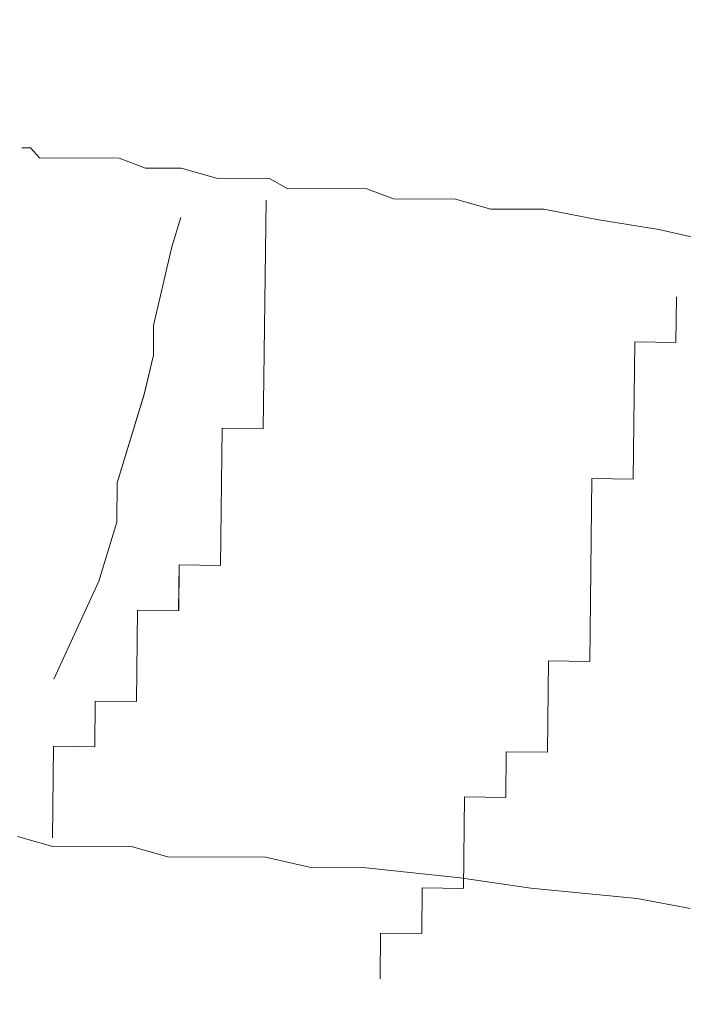
# Model space of a CAD drawing. Units: inches. Extents: x -466983 to 1020, y 324 to 318697.
# Tile 64 of 97: x 640.735 to 642.74, y 945.669 to 948.644. Entities that reach past the tile are written whole.
import ezdxf

# ---------------------------------------------------------------- set-up
doc = ezdxf.new("R2010")
doc.units = ezdxf.units.IN
doc.header["$MEASUREMENT"] = 0
doc.layers.add('A-FLOR-PATT', color=252, linetype='Continuous', lineweight=13)
doc.layers.add('A-FURN', color=8, linetype='Continuous', lineweight=18)

# ---------------------------------------------------------------- blocks, each defined once
blk = doc.blocks.new('L Shaped Sofa')
at = {"ltscale": 2}
for p, q in [((2422.3278, 737.9207), (2422.3309, 738.1726)), ((2422.0979, 737.6715), (2422.101, 737.9234)), ((2422.101, 737.9234), (2422.3278, 737.9207)), ((2420.6221, 737.7847), (2420.9145, 737.7291)), ((2420.9145, 737.7291), (2421.4997, 737.6721)), ((2421.4997, 737.6721), (2421.8898, 737.6161)), ((2421.8649, 737.1705), (2421.8711, 737.6743)), ((2421.8711, 737.6743), (2422.0979, 737.6715)), ((2421.8898, 737.6161), (2422.4262, 737.5593)), ((2422.4262, 737.5593), (2422.719, 737.558)), ((2422.719, 737.558), (2422.9626, 737.5026)), ((2422.9626, 737.5026), (2423.4994, 737.5001)), ((2423.4994, 737.5001), (2423.6942, 737.4449)), ((2423.6942, 737.4449), (2424.1334, 737.4429)), ((2424.1334, 737.4429), (2424.3282, 737.3878)), ((2424.1302, 736.8908), (2424.1364, 737.3947)), ((2421.635, 736.9213), (2421.6381, 737.1732)), ((2421.6381, 737.1732), (2421.8649, 737.1705)), ((2421.402, 736.4203), (2421.4082, 736.9241)), ((2421.4082, 736.9241), (2421.635, 736.9213)), ((2423.9003, 736.6417), (2423.9034, 736.8936)), ((2423.9034, 736.8936), (2424.1302, 736.8908)), ((2423.6673, 736.1406), (2423.6735, 736.6445)), ((2423.6735, 736.6445), (2423.9003, 736.6417)), ((2423.8804, 735.9802), (2424.1277, 736.5212)), ((2421.1629, 735.4154), (2421.1752, 736.423)), ((2421.1752, 736.423), (2421.402, 736.4203)), ((2423.4374, 735.8915), (2423.4405, 736.1434)), ((2423.4405, 736.1434), (2423.6673, 736.1406)), ((2423.7808, 735.6554), (2423.8804, 735.9802)), ((2423.2013, 735.1385), (2423.2106, 735.8943)), ((2423.2106, 735.8943), (2423.4374, 735.8915)), ((2423.7795, 735.4385), (2423.7808, 735.6554)), ((2420.9268, 734.6624), (2420.936, 735.4182)), ((2420.936, 735.4182), (2421.1629, 735.4154)), ((2423.6301, 734.9512), (2423.7795, 735.4385)), ((2422.9591, 733.8818), (2422.9745, 735.1413)), ((2422.9745, 735.1413), (2423.2013, 735.1385)), ((2423.58, 734.7346), (2423.6301, 734.9512)), ((2423.579, 734.572), (2423.58, 734.7346)), ((2420.6969, 734.4133), (2420.7, 734.6652)), ((2420.7, 734.6652), (2420.9268, 734.6624)), ((2423.4788, 734.1387), (2423.579, 734.572)), ((2423.429, 733.9763), (2423.4788, 734.1387)), ((2420.5507, 734.0982), (2420.7944, 734.0429)), ((2420.7944, 734.0429), (2421.1356, 733.987)), ((2421.1356, 733.987), (2421.428, 733.9315)), ((2421.428, 733.9315), (2421.7208, 733.9301)), ((2421.7208, 733.9301), (2421.9157, 733.8749)), ((2421.9157, 733.8749), (2422.2572, 733.8733)), ((2422.2572, 733.8733), (2422.4033, 733.8184)), ((2422.4033, 733.8184), (2422.8424, 733.8164)), ((2422.8424, 733.8164), (2422.9397, 733.7617)), ((2422.9397, 733.7617), (2423.2325, 733.7603)), ((2423.2325, 733.7603), (2423.4273, 733.7052)), ((2423.4273, 733.7052), (2423.6225, 733.7043)), ((2423.6225, 733.7043), (2423.7686, 733.6494)), ((2423.7686, 733.6494), (2424.2077, 733.6473)), ((2424.2077, 733.6473), (2424.2562, 733.5929)), ((2424.2562, 733.5929), (2424.305, 733.5926))]:
    blk.add_line(p, q, dxfattribs=at)

msp = doc.modelspace()

# ---------------------------------------------------------------- hatches: boundary and pattern name
at = {"layer": 'A-FLOR-PATT', "transparency": 33554572}
h = msp.add_hatch(dxfattribs=at)
h.set_pattern_fill('ANSI37', color=256, scale=30)
h.set_pattern_definition([(45, (-1212.4137, -290.035), (-2.6516504, 2.6516504), []), (135, (-1212.4137, -290.035), (-2.6516504, -2.6516504), [])])
h.paths.add_polyline_path([(901.8057, 1075.9377), (900.6144, 1075.9377), (900.6144, 1065.3856), (899.391, 1065.3856), (898.0911, 1065.3856), (892.8356, 1058.7098, -0.258377), (892.1875, 1058.3509), (879.9848, 1058.3509, -0.20177), (879.4382, 1058.5808), (874.0812, 1065.3856), (872.7813, 1065.3856), (871.5579, 1065.3856), (871.5579, 1075.9377), (813.8057, 1075.9377), (813.8057, 1044.7922), (832.3947, 1044.7922, -0.394795), (848.6602, 1028.5356), (848.6602, 1009.9377), (901.8057, 1009.9377), (901.8057, 1015.9377), (901.3057, 1015.9377), (871.3057, 1015.9377), (871.3057, 1017.2502), (871.3344, 1017.2502, -0.401453), (901.3057, 1045.9377), (901.8057, 1045.9377)])
edge = h.paths.add_edge_path(flags=16)
edge.add_line((847.7731, 1068.9486), (847.7731, 1073.7088))
edge.add_arc((849.2269, 1073.7088), 1.4538, 90, 180, ccw=False)
edge.add_line((849.2269, 1075.1627), (864.4921, 1075.1627))
edge.add_arc((864.4921, 1073.7088), 1.4538, 0, 90, ccw=False)
edge.add_line((865.9459, 1073.7088), (865.9459, 1069.0035))
edge.add_arc((832.6447, 1068.9761), 33.3012, -20.61234, 0.04725, ccw=False)
edge.add_ellipse((856.8595, 1058.48), major_axis=(0, 10.2131), ratio=0.6859192, start_angle=100.00884, end_angle=259.99116, ccw=False)
edge.add_arc((881.0742, 1068.9761), 33.3012, 180.04725, 200.61234, ccw=False)
h.paths.add_polyline_path([(853.1456, 1066.4815), (853.1456, 1066.4534), (853.1463, 1066.4534, 0.433107), (852.9166, 1066.6849), (852.9166, 1066.4534), (853.1456, 1066.4534), (853.1456, 1066.4815), (853.088, 1066.6122, 0.697939), (852.6995, 1066.4534), (852.7003, 1066.4534), (852.7003, 1066.4815), (852.9166, 1067.0012), (852.9166, 1066.6849, -0.396254)], flags=0)
h.paths.add_polyline_path([(861.0187, 1066.4815), (861.0187, 1066.4534), (861.0194, 1066.4534, 0.416404), (860.8024, 1066.6849), (860.8024, 1066.4534), (861.0187, 1066.4534), (861.0187, 1066.4815), (860.9672, 1066.6053, 0.713344), (860.5726, 1066.4534), (860.5734, 1066.4534), (860.5734, 1066.4815), (860.8024, 1067.0012), (860.8024, 1066.6849, -0.379973)], flags=0)
edge = h.paths.add_edge_path(flags=0)
edge.add_spline(control_points=[(861.1298, 1065.7855), (861.4661, 1065.2478), (861.6134, 1065.0161), (861.9833, 1064.3736), (862.1924, 1063.9443), (862.5614, 1063.0391), (862.7212, 1062.5633), (862.9865, 1061.5781), (863.092, 1061.0689), (863.2452, 1060.031), (863.293, 1059.5025), (863.3295, 1058.4409), (863.3181, 1057.9078), (863.2366, 1056.8518), (863.1664, 1056.3289), (862.9695, 1055.308), (862.8427, 1054.8099), (862.5365, 1053.8522), (862.3571, 1053.3927), (861.9514, 1052.5249), (861.7251, 1052.1166), (861.233, 1051.3622), (860.9672, 1051.0162), (860.4048, 1050.3949), (860.1082, 1050.1197), (859.4937, 1049.6461), (859.1758, 1049.4476), (858.5276, 1049.1299), (858.1973, 1049.0107), (857.5315, 1048.8518), (857.1959, 1048.8121), (856.5249, 1048.812), (856.1894, 1048.8515), (855.5236, 1049.0101), (855.1933, 1049.1291), (854.545, 1049.4465), (854.2271, 1049.6449), (853.6124, 1050.1183), (853.3158, 1050.3933), (852.7533, 1051.0143), (852.4874, 1051.3602), (851.9952, 1052.1144), (851.7688, 1052.5225), (851.3629, 1053.3902), (851.1834, 1053.8496), (850.877, 1054.8071), (850.7501, 1055.3051), (850.553, 1056.326), (850.4827, 1056.8488), (850.401, 1057.9048), (850.3895, 1058.4379), (850.4257, 1059.4995), (850.4734, 1060.0281), (850.6265, 1061.066), (850.7318, 1061.5753), (850.9969, 1062.5605), (851.1567, 1063.0365), (851.5254, 1063.9418), (851.7345, 1064.3712), (852.1056, 1065.0164), (852.2544, 1065.2503), (852.6082, 1065.7335)], knot_values=[3.915332, 3.915332, 3.915332, 3.915332, 4.013468, 4.013468, 4.175532, 4.175532, 4.337596, 4.337596, 4.49966, 4.49966, 4.661724, 4.661724, 4.823788, 4.823788, 4.985852, 4.985852, 5.147916, 5.147916, 5.30998, 5.30998, 5.472044, 5.472044, 5.634109, 5.634109, 5.796173, 5.796173, 5.958237, 5.958237, 6.120301, 6.120301, 6.282365, 6.282365, 6.444429, 6.444429, 6.606493, 6.606493, 6.768557, 6.768557, 6.930621, 6.930621, 7.092685, 7.092685, 7.254749, 7.254749, 7.416813, 7.416813, 7.578878, 7.578878, 7.740942, 7.740942, 7.903006, 7.903006, 8.06507, 8.06507, 8.227134, 8.227134, 8.389198, 8.389198, 8.551262, 8.551262, 8.65037, 8.65037, 8.65037, 8.65037], degree=3, periodic=0)
edge.add_line((852.6421, 1065.7855), (861.1298, 1065.7855))
edge = h.paths.add_edge_path(flags=0)
edge.add_ellipse((856.8496, 1057.7432), major_axis=(0, 7.7921), ratio=0.687861, start_angle=0, end_angle=360)
h.paths.add_polyline_path([(848.8634, 1069.3891), (848.8634, 1073.9605, -0.414214), (849.9538, 1075.0508), (863.7652, 1075.0508, -0.414214), (864.8555, 1073.9605), (864.8555, 1069.3891, -0.388936), (864.5237, 1069.027, -0.043561), (849.1953, 1069.027, -0.388936)], flags=0)
h.paths.add_polyline_path([(853.1006, 1068.1122, -1), (852.6775, 1068.1122, -1)], flags=0)
edge = h.paths.add_edge_path(flags=0)
edge.add_ellipse((856.8595, 1057.3378), major_axis=(0, 2.207), ratio=0.657164, start_angle=0, end_angle=360)
h.paths.add_polyline_path([(861.0415, 1068.1122, -1), (860.6184, 1068.1122, -1)], flags=0)
edge = h.paths.add_edge_path()
edge.add_line((573.9537, 1057.3412), (573.9537, 1075.9377))
edge.add_line((573.9537, 1075.9377), (558.7308, 1075.9377))
edge.add_line((558.7308, 1075.9377), (558.7308, 1065.3856))
edge.add_line((558.7308, 1065.3856), (557.5074, 1065.3856))
edge.add_line((557.5074, 1065.3856), (556.2075, 1065.3856))
edge.add_line((556.2075, 1065.3856), (550.952, 1058.7098))
edge.add_arc((550.3039, 1059.1155), 0.7646, 270, 327.9483, ccw=False)
edge.add_line((550.3039, 1058.3509), (538.1012, 1058.3509))
edge.add_arc((538.1012, 1059.1155), 0.7646, 224.3704, 270, ccw=False)
edge.add_line((537.5546, 1058.5808), (532.1976, 1065.3856))
edge.add_line((532.1976, 1065.3856), (530.8977, 1065.3856))
edge.add_line((530.8977, 1065.3856), (529.6743, 1065.3856))
edge.add_line((529.6743, 1065.3856), (529.6743, 1075.9377))
edge.add_line((529.6743, 1075.9377), (520.8057, 1075.9377))
edge.add_line((520.8057, 1075.9377), (520.8057, 1045.9377))
edge.add_line((520.8057, 1045.9377), (521.3057, 1045.9377))
edge.add_arc((521.3057, 1015.9377), 30, 2.50749, 90, ccw=False)
edge.add_line((551.277, 1017.2502), (551.3057, 1017.2502))
edge.add_line((551.3057, 1017.2502), (551.3057, 1015.9377))
edge.add_line((551.3057, 1015.9377), (520.8057, 1015.9377))
edge.add_line((520.8057, 1015.9377), (520.8057, 1009.9377))
edge.add_line((520.8057, 1009.9377), (559.1913, 1010.4022))
edge.add_arc((559.1913, 1011.856), 1.4538, 180, 270, ccw=False)
edge.add_line((557.7375, 1011.856), (557.7375, 1016.5613))
edge.add_arc((591.0386, 1016.5888), 33.3012, 159.38766, 180.04725, ccw=False)
edge.add_ellipse((566.8239, 1027.0848), major_axis=(0, 10.2131), ratio=0.6859192, start_angle=280.00884, end_angle=439.99116, ccw=False)
edge.add_arc((542.6091, 1016.5888), 33.3012, 0.04725, 20.61234, ccw=False)
edge.add_line((575.9103, 1016.6162), (575.9103, 1011.856))
edge.add_arc((574.4565, 1011.856), 1.4538, -90, 0, ccw=False)
edge.add_line((574.4565, 1010.4022), (608.8057, 1009.9377))
edge.add_line((608.8057, 1009.9377), (608.8057, 1041.0857))
edge.add_line((608.8057, 1041.0857), (590.2179, 1041.0857))
edge.add_arc((590.775, 1057.9074), 16.8309, 181.92775, 268.10321, ccw=False)
edge = h.paths.add_edge_path()
edge.add_ellipse((494.2443, 583.6204), major_axis=(0, 10.2131), ratio=0.6859192, start_angle=280.00884, end_angle=439.99116, ccw=False)
edge.add_arc((470.0296, 573.1243), 33.3012, 0.04725, 20.61234, ccw=False)
edge.add_line((503.3307, 573.1518), (503.3307, 568.3916))
edge.add_arc((501.8769, 568.3916), 1.4538, -90, 0, ccw=False)
edge.add_line((501.8769, 566.9377), (539.8057, 566.9377))
edge.add_line((539.8057, 566.9377), (539.8057, 572.9377))
edge.add_line((539.8057, 572.9377), (539.3057, 572.9377))
edge.add_line((539.3057, 572.9377), (509.3057, 572.9377))
edge.add_line((509.3057, 572.9377), (509.3057, 574.2502))
edge.add_line((509.3057, 574.2502), (509.3344, 574.2502))
edge.add_arc((539.3057, 572.9377), 30, 90, 177.49251, ccw=False)
edge.add_line((539.3057, 602.9377), (539.8057, 602.9377))
edge.add_line((539.8057, 602.9377), (539.8057, 626.9377))
edge.add_line((539.8057, 626.9377), (531.7718, 626.9377))
edge.add_line((531.7718, 626.9377), (531.7718, 616.3856))
edge.add_line((531.7718, 616.3856), (530.5484, 616.3856))
edge.add_line((530.5484, 616.3856), (529.2485, 616.3856))
edge.add_line((529.2485, 616.3856), (523.7105, 609.3509))
edge.add_line((523.7105, 609.3509), (510.7766, 609.3509))
edge.add_line((510.7766, 609.3509), (505.2386, 616.3856))
edge.add_line((505.2386, 616.3856), (503.9387, 616.3856))
edge.add_line((503.9387, 616.3856), (502.7153, 616.3856))
edge.add_line((502.7153, 616.3856), (502.7153, 626.9377))
edge.add_line((502.7153, 626.9377), (481.6983, 626.9377))
edge.add_line((481.6983, 626.9377), (481.6983, 610.995))
edge.add_arc((467.2703, 611.4728), 14.4359, 271.92775, 358.10321, ccw=False)
edge.add_line((467.7559, 597.0451), (451.8057, 597.0451))
edge.add_line((451.8057, 597.0451), (451.8057, 584.4035))
edge.add_line((451.8057, 584.4035), (451.8057, 566.9377))
edge.add_line((451.8057, 566.9377), (486.6117, 566.9377))
edge.add_arc((486.6117, 568.3916), 1.4538, 180, 270, ccw=False)
edge.add_line((485.1579, 568.3916), (485.1579, 573.0969))
edge.add_arc((518.4591, 573.1243), 33.3012, 159.38766, 180.04725, ccw=False)
h.paths.add_polyline_path([(836.2609, 1020.7328), (879.8898, 1020.7328), (879.8898, 1039.3902), (836.2609, 1039.3902)], flags=25)
h.paths.add_polyline_path([(549.9851, 1036.7492), (593.614, 1036.7492), (593.614, 1055.4065), (549.9851, 1055.4065)], flags=24)
h.paths.add_polyline_path([(475.123, 595.5959), (518.752, 595.5959), (518.752, 614.2532), (475.123, 614.2532)], flags=24)
h = msp.add_hatch(dxfattribs=at)
h.set_pattern_fill('ANSI37', color=256, scale=20)
h.set_pattern_definition([(45, (-1212.4137, -290.035), (-1.767767, 1.767767), []), (135, (-1212.4137, -290.035), (-1.767767, -1.767767), [])])
h.paths.add_polyline_path([(809.8057, 870.9377), (809.8057, 888.1519), (806.9985, 888.1519), (802.6624, 888.1519), (789.3832, 888.1519), (786.2846, 888.1519, -0.414214), (785.4991, 888.9374), (785.4991, 900.1959), (785.4991, 908.4696, -0.414214), (786.8082, 909.7787, -0.414214), (785.4991, 911.0878), (785.4991, 929.1015, -0.414214), (786.8082, 930.4106, -0.414214), (785.4991, 931.7197), (785.4991, 931.9039, -0.414214), (784.19, 930.5948), (766.7223, 930.5948, -0.412359), (765.4132, 931.8956, -0.413741), (764.1145, 930.5782), (744.5781, 930.422, -0.416556), (743.7864, 931.2075), (743.7864, 933.5153), (742.2154, 933.5153), (742.2154, 952.024, -0.001344), (743.7864, 952.1998), (743.7864, 953.9377), (678.5915, 953.9377), (678.5915, 951.1305), (678.5915, 946.7945), (678.5915, 933.5153), (678.5915, 930.4166, -0.414214), (677.806, 929.6312), (666.5475, 929.6312), (658.2738, 929.6312, -0.414214), (656.9647, 930.9403, -0.414214), (655.6556, 929.6312), (637.6419, 929.6312, -0.414214), (636.3328, 930.9403, -0.414214), (635.0237, 929.6312), (634.8395, 929.6312, -0.414214), (636.1486, 928.322), (636.1486, 910.8544, -0.412359), (634.8478, 909.5452, -0.413741), (636.1653, 908.2466), (636.3214, 888.7102, -0.416556), (635.5359, 887.9184), (633.2281, 887.9184), (633.2281, 886.3475), (614.7194, 886.3475, -0.001344), (614.5436, 887.9184), (612.8057, 887.9184), (612.8057, 834.9377), (612.8057, 752.9377), (612.8057, 748.9377), (612.8057, 697.9377), (654.8057, 697.9377), (654.8057, 701.9377), (715.8057, 701.9377), (715.8057, 737.4353), (774.2918, 737.4353), (774.2918, 795.9377), (809.8057, 795.9377)])
h.paths.add_polyline_path([(679.2761, 849.5757, 0.102523), (682.1475, 849.2608, -0.080461), (694.5428, 849.7725, -0.283899), (694.4822, 849.0082, 0.136605), (694.4068, 848.8103, -0.030441), (694.5428, 846.8929), (694.5428, 842.6198), (694.5428, 838.3466, -0.028219), (694.4246, 836.5684), (694.425, 836.5684, 0.196187), (694.4456, 836.2708, -0.302897), (694.5428, 835.467, -0.080461), (682.1475, 835.9787, 0.102523), (679.2761, 835.6638, -0.58611), (678.6457, 836.0169), (678.6457, 849.2227, -0.58611)], flags=16)
h.paths.add_polyline_path([(679.5173, 848.6515, 0.699597), (679.476, 848.6342, 1.20716), (679.1935, 848.7422, 0.010621)], flags=0)
h.paths.add_polyline_path([(679.4923, 836.5608, -0.013798), (679.9178, 836.6594, -0.071703), (682.8533, 837.1434, -0.165743), (682.1665, 839.1006), (682.1665, 842.6094), (682.1665, 846.0603, -0.240616), (683.4733, 848.6767, -0.068263), (693.9295, 849.0082), (693.7875, 848.7083), (693.7875, 849.0228, 0.067332), (683.4733, 848.6767, 0.240616), (682.1665, 846.0603), (682.1665, 842.6094), (682.1665, 839.1006, 0.23459), (683.461, 836.5513, 0.068093), (693.7875, 836.1955), (693.7875, 836.5104), (693.9296, 836.2102, -0.077215), (682.2421, 836.7815, 0.086627), (679.5283, 836.5701, -0.628402), (679.5029, 836.5735), (679.5029, 836.6071, 0.910458)], flags=0)
h.paths.add_polyline_path([(679.476, 848.6364), (679.2069, 848.647), (679.2069, 836.5718, 0.913566), (679.3645, 836.5861), (679.476, 836.5824)], flags=0)
h.paths.add_polyline_path([(679.2761, 829.8604, 0.102523), (682.1475, 829.5455, -0.080461), (694.5428, 830.0572, -0.283899), (694.4822, 829.2929, 0.136605), (694.4068, 829.095, -0.030441), (694.5428, 827.1776), (694.5428, 822.9045), (694.5428, 818.6314, -0.028219), (694.4246, 816.8531), (694.425, 816.8532, 0.196187), (694.4456, 816.5555, -0.302897), (694.5428, 815.7517, -0.080461), (682.1475, 816.2635, 0.102523), (679.2761, 815.9485, -0.58611), (678.6457, 816.3016), (678.6457, 829.5074, -0.58611)], flags=16)
h.paths.add_polyline_path([(679.5173, 828.9362, 0.699597), (679.476, 828.9189, 1.20716), (679.1935, 829.0269, 0.010621)], flags=0)
h.paths.add_polyline_path([(679.4923, 816.8456, -0.013798), (679.9178, 816.9441, -0.071703), (682.8533, 817.4281, -0.165743), (682.1665, 819.3853), (682.1665, 822.8941), (682.1665, 826.345, -0.240616), (683.4733, 828.9614, -0.068263), (693.9295, 829.2929), (693.7875, 828.9931), (693.7875, 829.3076, 0.067332), (683.4733, 828.9614, 0.240616), (682.1665, 826.345), (682.1665, 822.8941), (682.1665, 819.3853, 0.23459), (683.461, 816.836, 0.068093), (693.7875, 816.4802), (693.7875, 816.7952), (693.9296, 816.4949, -0.077215), (682.2421, 817.0662, 0.086627), (679.5283, 816.8549, -0.628402), (679.5029, 816.8582), (679.5029, 816.8918, 0.910458)], flags=0)
h.paths.add_polyline_path([(679.476, 828.9211), (679.2069, 828.9317), (679.2069, 816.8565, 0.913566), (679.3645, 816.8708), (679.476, 816.8671)], flags=0)
h.paths.add_polyline_path([(679.2761, 810.1451, 0.102523), (682.1475, 809.8302, -0.080461), (694.5428, 810.342, -0.3023), (694.4466, 809.5394, 0.10023), (694.4058, 809.3878, -0.03057), (694.5428, 807.4623), (694.5428, 803.1892), (694.5428, 798.9161, -0.03057), (694.4058, 796.9906, 0.10023), (694.4466, 796.839, -0.3023), (694.5428, 796.0365, -0.080461), (682.1475, 796.5482, 0.102523), (679.2761, 796.2333, -0.58611), (678.6457, 796.5863), (678.6457, 809.7921, -0.58611)], flags=16)
h.paths.add_polyline_path([(679.5173, 809.2417, 0.699597), (679.476, 809.2244, 1.20716), (679.1935, 809.3324, 0.010621)], flags=0)
h.paths.add_polyline_path([(679.4923, 797.151, -0.013798), (679.9178, 797.2496, -0.071703), (682.8533, 797.7336, -0.165743), (682.1665, 799.6908), (682.1665, 803.1996), (682.1665, 806.6505, -0.239349), (683.461, 809.2577, -0.072465), (694.4468, 809.5405, 0.197932), (694.425, 809.2405), (693.7875, 809.2985), (693.7875, 809.6135, 0.068093), (683.461, 809.2577, 0.239349), (682.1665, 806.6505), (682.1665, 803.1996), (682.1665, 799.6908, 0.235854), (683.4733, 797.1323, 0.067332), (693.7875, 796.7861), (693.7875, 797.1006), (694.425, 797.1586, 0.197932), (694.4468, 796.8586, -0.080419), (682.1557, 797.3795, 0.083867), (679.5283, 797.1603, -0.628402), (679.5029, 797.1637), (679.5029, 797.1973, 0.910458)], flags=0)
h.paths.add_polyline_path([(679.2069, 809.2372), (679.2069, 797.162, 0.913566), (679.3645, 797.1763), (679.476, 797.1726), (679.476, 809.2266)], flags=0)
h.paths.add_polyline_path([(695.3643, 853.2989), (728.2231, 853.2989), (728.2231, 771.1519), (695.3643, 771.1519)], flags=16)
h.paths.add_polyline_path([(696.0215, 852.6417), (727.5659, 852.6417), (727.5659, 771.809), (696.0215, 771.809)], flags=0)
h.paths.add_polyline_path([(679.2761, 788.7869, 0.102523), (682.1475, 788.472, -0.080461), (694.5428, 788.9837, -0.3023), (694.4466, 788.1812, 0.10023), (694.4058, 788.0296, -0.03057), (694.5428, 786.1041), (694.5428, 781.831), (694.5428, 777.5578, -0.03057), (694.4058, 775.6323, 0.10023), (694.4466, 775.4808, -0.3023), (694.5428, 774.6782, -0.080461), (682.1475, 775.19, 0.102523), (679.2761, 774.875, -0.58611), (678.6457, 775.2281), (678.6457, 788.4339, -0.58611)], flags=16)
h.paths.add_polyline_path([(679.5173, 787.8834, 0.699597), (679.476, 787.8662, 1.20716), (679.1935, 787.9742, 0.010621)], flags=0)
h.paths.add_polyline_path([(679.4923, 775.7928, -0.013798), (679.9178, 775.8914, -0.071703), (682.8533, 776.3753, -0.165743), (682.1665, 778.3325), (682.1665, 781.8414), (682.1665, 785.2922, -0.239349), (683.461, 787.8995, -0.072465), (694.4468, 788.1823, 0.197932), (694.425, 787.8823), (693.7875, 787.9403), (693.7875, 788.2553, 0.068093), (683.461, 787.8995, 0.239349), (682.1665, 785.2922), (682.1665, 781.8414), (682.1665, 778.3325, 0.235854), (683.4733, 775.7741, 0.067332), (693.7875, 775.4279), (693.7875, 775.7424), (694.425, 775.8004, 0.197932), (694.4468, 775.5004, -0.080419), (682.1557, 776.0212, 0.083867), (679.5283, 775.8021, -0.628402), (679.5029, 775.8054), (679.5029, 775.8391, 0.910458)], flags=0)
h.paths.add_polyline_path([(679.2069, 787.8789), (679.2069, 775.8038, 0.913566), (679.3645, 775.818), (679.476, 775.8144), (679.476, 787.8684)], flags=0)
h.paths.add_polyline_path([(704.641, 854.1204, -0.080461), (705.1527, 866.5157, 0.102523), (704.8378, 869.3871, -0.58611), (705.1908, 870.0174), (718.3966, 870.0174, -0.58611), (718.7496, 869.3871, 0.102523), (718.4347, 866.5157, -0.080461), (718.9465, 854.1204, -0.3023), (718.1439, 854.2166, 0.10023), (717.9924, 854.2574, -0.03057), (716.0668, 854.1204), (711.7937, 854.1204), (707.5206, 854.1204, -0.03057), (705.5951, 854.2574, 0.10023), (705.4435, 854.2166, -0.3023)], flags=16)
h.paths.add_polyline_path([(717.8462, 869.1459, 0.699597), (717.8289, 869.1872, 1.20716), (717.9369, 869.4697, 0.010621)], flags=0)
h.paths.add_polyline_path([(705.4631, 854.2164, -0.080419), (705.984, 866.5074, 0.083867), (705.7648, 869.1349, -0.628402), (705.7682, 869.1603), (705.8018, 869.1603, 0.910458), (705.7555, 869.1709, -0.013798), (705.8541, 868.7454, -0.071703), (706.3381, 865.8099, -0.165743), (708.2953, 866.4967), (711.8041, 866.4967), (715.255, 866.4967, -0.239349), (717.8622, 865.2022, -0.072465), (718.145, 854.2164, 0.197932), (717.845, 854.2382), (717.903, 854.8757), (718.218, 854.8757, 0.068093), (717.8622, 865.2022, 0.239349), (715.255, 866.4967), (711.8041, 866.4967), (708.2953, 866.4967, 0.235854), (705.7368, 865.1898, 0.067332), (705.3906, 854.8757), (705.7051, 854.8757), (705.7631, 854.2382, 0.197932)], flags=16)
h.paths.add_polyline_path([(705.7665, 869.4563, 0.913566), (705.7808, 869.2987), (705.7771, 869.1872), (717.8311, 869.1872), (717.8417, 869.4563)], flags=0)
h.paths.add_polyline_path([(729.0446, 842.6198), (729.0446, 846.8929, -0.03057), (729.1817, 848.8184, 0.10023), (729.1408, 848.9699, -0.3023), (729.0446, 849.7725, -0.080461), (741.4399, 849.2608, 0.102523), (744.3113, 849.5757, -0.58611), (744.9417, 849.2227), (744.9417, 836.0169, -0.58611), (744.3113, 835.6638, 0.102523), (741.4399, 835.9787, -0.080461), (729.0446, 835.467, -0.3023), (729.1408, 836.2696, 0.10023), (729.1817, 836.4211, -0.03057), (729.0446, 838.3466)], flags=16)
h.paths.add_polyline_path([(744.1115, 836.5846, 1.20716), (744.3939, 836.4766, 0.010621), (744.0701, 836.5673, 0.699597)], flags=0)
h.paths.add_polyline_path([(729.1407, 836.2684, 0.197932), (729.1624, 836.5684), (729.7999, 836.5104), (729.7999, 836.1955, 0.068093), (740.1264, 836.5513, 0.239349), (741.4209, 839.1585), (741.4209, 842.6094), (741.4209, 846.1182, 0.235854), (740.1141, 848.6767, 0.067332), (729.7999, 849.0228), (729.7999, 848.7083), (729.1624, 848.6503, 0.197932), (729.1407, 848.9504, -0.080419), (741.4317, 848.4295, 0.083867), (744.0591, 848.6486, -0.628402), (744.0845, 848.6453), (744.0845, 848.6117, 0.910458), (744.0951, 848.6579, -0.013798), (743.6696, 848.5594, -0.071703), (740.7341, 848.0754, -0.165743), (741.4209, 846.1182), (741.4209, 842.6094), (741.4209, 839.1585, -0.239349), (740.1264, 836.5513, -0.072465)], flags=0)
h.paths.add_polyline_path([(729.0446, 830.0572, -0.080461), (741.4399, 829.5455, 0.102523), (744.3113, 829.8604, -0.58611), (744.9417, 829.5074), (744.9417, 816.3016, -0.58611), (744.3113, 815.9485, 0.102523), (741.4399, 816.2635, -0.080461), (729.0446, 815.7517, -0.3023), (729.1408, 816.5543, 0.10023), (729.1817, 816.7058, -0.03057), (729.0446, 818.6314), (729.0446, 822.9045), (729.0446, 827.1776, -0.03057), (729.1817, 829.1031, 0.10023), (729.1408, 829.2547, -0.3023)], flags=16)
h.paths.add_polyline_path([(744.1115, 816.8693, 1.20716), (744.3939, 816.7613, 0.010621), (744.0701, 816.852, 0.699597)], flags=0)
h.paths.add_polyline_path([(729.1407, 829.2351, -0.080419), (741.4317, 828.7142, 0.083867), (744.0591, 828.9334, -0.628402), (744.0845, 828.93), (744.0845, 828.8964, 0.910458), (744.0951, 828.9427, -0.013798), (743.6696, 828.8441, -0.071703), (740.7341, 828.3601, -0.165743), (741.4209, 826.4029), (741.4209, 822.8941), (741.4209, 819.4432, -0.239349), (740.1264, 816.836, -0.072465), (729.1407, 816.5531, 0.197932), (729.1624, 816.8532), (729.7999, 816.7952), (729.7999, 816.4802, 0.068093), (740.1264, 816.836, 0.239349), (741.4209, 819.4432), (741.4209, 822.8941), (741.4209, 826.4029, 0.235854), (740.1141, 828.9614, 0.067332), (729.7999, 829.3076), (729.7999, 828.9931), (729.1624, 828.9351, 0.197932)], flags=16)
h.paths.add_polyline_path([(729.0446, 810.342, -0.080461), (741.4399, 809.8302, 0.102523), (744.3113, 810.1451, -0.58611), (744.9417, 809.7921), (744.9417, 796.5863, -0.58611), (744.3113, 796.2333, 0.102523), (741.4399, 796.5482, -0.080461), (729.0446, 796.0365, -0.283899), (729.1052, 796.8007, 0.136605), (729.1806, 796.9987, -0.030441), (729.0446, 798.9161), (729.0446, 803.1892), (729.0446, 807.4623, -0.028219), (729.1628, 809.2406), (729.1624, 809.2405, 0.196187), (729.1418, 809.5382, -0.302897)], flags=16)
h.paths.add_polyline_path([(744.1115, 797.1748, 1.20716), (744.3939, 797.0668, 0.010621), (744.0701, 797.1575, 0.699597)], flags=0)
h.paths.add_polyline_path([(741.3453, 809.0275, 0.086627), (744.0591, 809.2388, -0.628402), (744.0845, 809.2355), (744.0845, 809.2019, 0.910458), (744.0951, 809.2481, -0.013798), (743.6696, 809.1496, -0.071703), (740.7341, 808.6656, -0.165743), (741.4209, 806.7084), (741.4209, 803.1996), (741.4209, 799.7487, -0.240616), (740.1141, 797.1323, -0.068263), (729.658, 796.8008), (729.7999, 797.1006), (729.7999, 796.7861, 0.067332), (740.1141, 797.1323, 0.240616), (741.4209, 799.7487), (741.4209, 803.1996), (741.4209, 806.7084, 0.23459), (740.1264, 809.2577, 0.068093), (729.7999, 809.6135), (729.7999, 809.2985), (729.6578, 809.5988, -0.077215)], flags=0)
h.paths.add_polyline_path([(704.641, 770.3304, -0.283899), (705.4053, 770.2697, 0.136605), (705.6032, 770.1944, -0.030441), (707.5206, 770.3304), (711.7937, 770.3304), (716.0668, 770.3304, -0.028219), (717.8451, 770.2122), (717.845, 770.2126, 0.196187), (718.1427, 770.2331, -0.302897), (718.9465, 770.3304, -0.080461), (718.4347, 757.9351, 0.102523), (718.7496, 755.0637, -0.58611), (718.3966, 754.4333), (705.1908, 754.4333, -0.58611), (704.8378, 755.0637, 0.102523), (705.1527, 757.9351, -0.080461)], flags=16)
h.paths.add_polyline_path([(705.762, 755.3048, 0.699597), (705.7793, 755.2635, 1.20716), (705.6713, 754.9811, 0.010621)], flags=0)
h.paths.add_polyline_path([(705.4053, 769.717), (705.7051, 769.5751), (705.3906, 769.5751, 0.067332), (705.7368, 759.2609, 0.240616), (708.3532, 757.954), (711.8041, 757.954), (715.3129, 757.954, 0.23459), (717.8622, 759.2485, 0.068093), (718.218, 769.5751), (717.903, 769.5751), (718.2033, 769.7172, -0.077215), (717.632, 758.0297, 0.086627), (717.8433, 755.3159, -0.628402), (717.84, 755.2904), (717.8064, 755.2904, 0.910458), (717.8526, 755.2799, -0.013798), (717.7541, 755.7053, -0.071703), (717.2701, 758.6409, -0.165743), (715.3129, 757.954), (711.8041, 757.954), (708.3532, 757.954, -0.240616), (705.7368, 759.2609, -0.068263)], flags=0)
h.paths.add_polyline_path([(729.0446, 788.9837, -0.080461), (741.4399, 788.472, 0.102523), (744.3113, 788.7869, -0.58611), (744.9417, 788.4339), (744.9417, 775.2281, -0.58611), (744.3113, 774.875, 0.102523), (741.4399, 775.19, -0.080461), (729.0446, 774.6782, -0.283899), (729.1052, 775.4425, 0.136605), (729.1806, 775.6405, -0.030441), (729.0446, 777.5578), (729.0446, 781.831), (729.0446, 786.1041, -0.028219), (729.1628, 787.8823), (729.1624, 787.8823, 0.196187), (729.1418, 788.1799, -0.302897)], flags=16)
h.paths.add_polyline_path([(744.1115, 775.8165, 1.20716), (744.3939, 775.7086, 0.010621), (744.0701, 775.7993, 0.699597)], flags=0)
h.paths.add_polyline_path([(741.3453, 787.6692, 0.086627), (744.0591, 787.8806, -0.628402), (744.0845, 787.8773), (744.0845, 787.8437, 0.910458), (744.0951, 787.8899, -0.013798), (743.6696, 787.7913, -0.071703), (740.7341, 787.3074, -0.165743), (741.4209, 785.3502), (741.4209, 781.8414), (741.4209, 778.3905, -0.240616), (740.1141, 775.7741, -0.068263), (729.658, 775.4425), (729.7999, 775.7424), (729.7999, 775.4279, 0.067332), (740.1141, 775.7741, 0.240616), (741.4209, 778.3905), (741.4209, 781.8414), (741.4209, 785.3502, 0.23459), (740.1264, 787.8995, 0.068093), (729.7999, 788.2553), (729.7999, 787.9403), (729.6578, 788.2405, -0.077215)], flags=0)
h.paths.add_polyline_path([(744.1115, 848.6364), (744.1115, 836.5824), (744.3805, 836.5718), (744.3805, 848.647, 0.913566), (744.2229, 848.6327)], flags=0)
h.paths.add_polyline_path([(744.2229, 828.9174), (744.1115, 828.9211), (744.1115, 816.8671), (744.3805, 816.8565), (744.3805, 828.9317, 0.913566)], flags=0)
h.paths.add_polyline_path([(717.8311, 755.2635), (705.7771, 755.2635), (705.7665, 754.9945), (717.8417, 754.9945, 0.913566), (717.8274, 755.1521)], flags=0)
h.paths.add_polyline_path([(744.2229, 809.2229), (744.1115, 809.2266), (744.1115, 797.1726), (744.3805, 797.162), (744.3805, 809.2372, 0.913566)], flags=0)
h.paths.add_polyline_path([(744.1115, 787.8684), (744.1115, 775.8144), (744.3805, 775.8038), (744.3805, 787.8789, 0.913566), (744.2229, 787.8647)], flags=0)
h.paths.add_polyline_path([(678.8774, 877.1228), (737.6127, 877.1228), (737.6127, 899.5116), (678.8774, 899.5116)], flags=24)

# ---------------------------------------------------------------- linework, layer by layer
at = {"layer": 'A-FURN', "ltscale": 2}
for p, q in [((640.7683, 948.2563), (640.7415, 948.2564)), ((640.7683, 948.2563), (640.7415, 948.2564)), ((640.7683, 948.2563), (640.7415, 948.2564)), ((640.7683, 948.2563), (640.7415, 948.2564)), ((640.7683, 948.2563), (640.7415, 948.2564)), ((640.7683, 948.2563), (640.7415, 948.2564)), ((640.7949, 948.2265), (640.7683, 948.2563)), ((640.7949, 948.2265), (640.7683, 948.2563)), ((640.7949, 948.2265), (640.7683, 948.2563)), ((640.7949, 948.2265), (640.7683, 948.2563)), ((640.7949, 948.2265), (640.7683, 948.2563)), ((640.7949, 948.2265), (640.7683, 948.2563)), ((641.0356, 948.2253), (640.7949, 948.2265)), ((641.0356, 948.2253), (640.7949, 948.2265)), ((641.0356, 948.2253), (640.7949, 948.2265)), ((641.0356, 948.2253), (640.7949, 948.2265)), ((641.0356, 948.2253), (640.7949, 948.2265)), ((641.0356, 948.2253), (640.7949, 948.2265)), ((641.1157, 948.1952), (641.0356, 948.2253)), ((641.1157, 948.1952), (641.0356, 948.2253)), ((641.1157, 948.1952), (641.0356, 948.2253)), ((641.1157, 948.1952), (641.0356, 948.2253)), ((641.1157, 948.1952), (641.0356, 948.2253)), ((641.1157, 948.1952), (641.0356, 948.2253)), ((641.2227, 948.1947), (641.1157, 948.1952)), ((641.2227, 948.1947), (641.1157, 948.1952)), ((641.2227, 948.1947), (641.1157, 948.1952)), ((641.2227, 948.1947), (641.1157, 948.1952)), ((641.2227, 948.1947), (641.1157, 948.1952)), ((641.2227, 948.1947), (641.1157, 948.1952)), ((641.3295, 948.1645), (641.2227, 948.1947)), ((641.3295, 948.1645), (641.2227, 948.1947)), ((641.3295, 948.1645), (641.2227, 948.1947)), ((641.3295, 948.1645), (641.2227, 948.1947)), ((641.3295, 948.1645), (641.2227, 948.1947)), ((641.3295, 948.1645), (641.2227, 948.1947)), ((641.49, 948.1638), (641.3295, 948.1645)), ((641.49, 948.1638), (641.3295, 948.1645)), ((641.49, 948.1638), (641.3295, 948.1645)), ((641.49, 948.1638), (641.3295, 948.1645)), ((641.49, 948.1638), (641.3295, 948.1645)), ((641.49, 948.1638), (641.3295, 948.1645)), ((641.5433, 948.1338), (641.49, 948.1638)), ((641.5433, 948.1338), (641.49, 948.1638)), ((641.5433, 948.1338), (641.49, 948.1638)), ((641.5433, 948.1338), (641.49, 948.1638)), ((641.5433, 948.1338), (641.49, 948.1638)), ((641.5433, 948.1338), (641.49, 948.1638)), ((641.7841, 948.1327), (641.5433, 948.1338)), ((641.7841, 948.1327), (641.5433, 948.1338)), ((641.7841, 948.1327), (641.5433, 948.1338)), ((641.7841, 948.1327), (641.5433, 948.1338)), ((641.7841, 948.1327), (641.5433, 948.1338)), ((641.7841, 948.1327), (641.5433, 948.1338)), ((641.8641, 948.1026), (641.7841, 948.1327)), ((641.8641, 948.1026), (641.7841, 948.1327)), ((641.8641, 948.1026), (641.7841, 948.1327)), ((641.8641, 948.1026), (641.7841, 948.1327)), ((641.8641, 948.1026), (641.7841, 948.1327)), ((641.8641, 948.1026), (641.7841, 948.1327)), ((642.0514, 948.1017), (641.8641, 948.1026)), ((642.0514, 948.1017), (641.8641, 948.1026)), ((642.0514, 948.1017), (641.8641, 948.1026)), ((642.0514, 948.1017), (641.8641, 948.1026)), ((642.0514, 948.1017), (641.8641, 948.1026)), ((642.0514, 948.1017), (641.8641, 948.1026)), ((642.1582, 948.0715), (642.0514, 948.1017)), ((642.1582, 948.0715), (642.0514, 948.1017)), ((642.1582, 948.0715), (642.0514, 948.1017)), ((642.1582, 948.0715), (642.0514, 948.1017)), ((642.1582, 948.0715), (642.0514, 948.1017)), ((642.1582, 948.0715), (642.0514, 948.1017)), ((641.4794, 948.098), (641.4709, 947.4074)), ((641.4794, 948.098), (641.4709, 947.4074)), ((641.4794, 948.098), (641.4709, 947.4074)), ((641.4794, 948.098), (641.4709, 947.4074)), ((641.4794, 948.098), (641.4709, 947.4074)), ((641.4794, 948.098), (641.4709, 947.4074)), ((642.3187, 948.0707), (642.1582, 948.0715)), ((642.3187, 948.0707), (642.1582, 948.0715)), ((642.3187, 948.0707), (642.1582, 948.0715)), ((642.3187, 948.0707), (642.1582, 948.0715)), ((642.3187, 948.0707), (642.1582, 948.0715)), ((642.3187, 948.0707), (642.1582, 948.0715)), ((642.479, 948.0402), (642.3187, 948.0707)), ((642.479, 948.0402), (642.3187, 948.0707)), ((642.479, 948.0402), (642.3187, 948.0707)), ((642.479, 948.0402), (642.3187, 948.0707)), ((642.479, 948.0402), (642.3187, 948.0707)), ((642.479, 948.0402), (642.3187, 948.0707)), ((641.2218, 948.0461), (641.1945, 947.9571)), ((641.2218, 948.0461), (641.1945, 947.9571)), ((641.2218, 948.0461), (641.1945, 947.9571)), ((641.2218, 948.0461), (641.1945, 947.9571)), ((641.2218, 948.0461), (641.1945, 947.9571)), ((641.2218, 948.0461), (641.1945, 947.9571)), ((642.6661, 948.0096), (642.479, 948.0402)), ((642.6661, 948.0096), (642.479, 948.0402)), ((642.6661, 948.0096), (642.479, 948.0402)), ((642.6661, 948.0096), (642.479, 948.0402)), ((642.6661, 948.0096), (642.479, 948.0402)), ((642.6661, 948.0096), (642.479, 948.0402)), ((642.7997, 947.9793), (642.6661, 948.0096)), ((642.7997, 947.9793), (642.6661, 948.0096)), ((642.7997, 947.9793), (642.6661, 948.0096)), ((642.7997, 947.9793), (642.6661, 948.0096)), ((642.7997, 947.9793), (642.6661, 948.0096)), ((642.7997, 947.9793), (642.6661, 948.0096)), ((641.1945, 947.9571), (641.1395, 947.7196)), ((641.1945, 947.9571), (641.1395, 947.7196)), ((641.1945, 947.9571), (641.1395, 947.7196)), ((641.1945, 947.9571), (641.1395, 947.7196)), ((641.1945, 947.9571), (641.1395, 947.7196)), ((641.1945, 947.9571), (641.1395, 947.7196)), ((642.7196, 947.8066), (642.7179, 947.6685)), ((642.7196, 947.8066), (642.7179, 947.6685)), ((642.7196, 947.8066), (642.7179, 947.6685)), ((642.7196, 947.8066), (642.7179, 947.6685)), ((642.7196, 947.8066), (642.7179, 947.6685)), ((642.7196, 947.8066), (642.7179, 947.6685)), ((641.1395, 947.7196), (641.139, 947.6304)), ((641.1395, 947.7196), (641.139, 947.6304)), ((641.1395, 947.7196), (641.139, 947.6304)), ((641.1395, 947.7196), (641.139, 947.6304)), ((641.1395, 947.7196), (641.139, 947.6304)), ((641.1395, 947.7196), (641.139, 947.6304)), ((642.5935, 947.67), (642.5884, 947.2557)), ((642.5935, 947.67), (642.5884, 947.2557)), ((642.5935, 947.67), (642.5884, 947.2557)), ((642.5935, 947.67), (642.5884, 947.2557)), ((642.5935, 947.67), (642.5884, 947.2557)), ((642.5935, 947.67), (642.5884, 947.2557)), ((642.7179, 947.6685), (642.5935, 947.67)), ((642.7179, 947.6685), (642.5935, 947.67)), ((642.7179, 947.6685), (642.5935, 947.67)), ((642.7179, 947.6685), (642.5935, 947.67)), ((642.7179, 947.6685), (642.5935, 947.67)), ((642.7179, 947.6685), (642.5935, 947.67)), ((641.139, 947.6304), (641.1115, 947.5116)), ((641.139, 947.6304), (641.1115, 947.5116)), ((641.139, 947.6304), (641.1115, 947.5116)), ((641.139, 947.6304), (641.1115, 947.5116)), ((641.139, 947.6304), (641.1115, 947.5116)), ((641.139, 947.6304), (641.1115, 947.5116)), ((641.1115, 947.5116), (641.0296, 947.2445)), ((641.1115, 947.5116), (641.0296, 947.2445)), ((641.1115, 947.5116), (641.0296, 947.2445)), ((641.1115, 947.5116), (641.0296, 947.2445)), ((641.1115, 947.5116), (641.0296, 947.2445)), ((641.1115, 947.5116), (641.0296, 947.2445)), ((641.3466, 947.409), (641.3415, 946.9947)), ((641.3466, 947.409), (641.3415, 946.9947)), ((641.3466, 947.409), (641.3415, 946.9947)), ((641.3466, 947.409), (641.3415, 946.9947)), ((641.3466, 947.409), (641.3415, 946.9947)), ((641.3466, 947.409), (641.3415, 946.9947)), ((641.4709, 947.4074), (641.3466, 947.409)), ((641.4709, 947.4074), (641.3466, 947.409)), ((641.4709, 947.4074), (641.3466, 947.409)), ((641.4709, 947.4074), (641.3466, 947.409)), ((641.4709, 947.4074), (641.3466, 947.409)), ((641.4709, 947.4074), (641.3466, 947.409)), ((641.0296, 947.2445), (641.0289, 947.1256)), ((641.0296, 947.2445), (641.0289, 947.1256)), ((641.0296, 947.2445), (641.0289, 947.1256)), ((641.0296, 947.2445), (641.0289, 947.1256)), ((641.0296, 947.2445), (641.0289, 947.1256)), ((641.0296, 947.2445), (641.0289, 947.1256)), ((642.4641, 947.2572), (642.4573, 946.7048)), ((642.4641, 947.2572), (642.4573, 946.7048)), ((642.4641, 947.2572), (642.4573, 946.7048)), ((642.4641, 947.2572), (642.4573, 946.7048)), ((642.4641, 947.2572), (642.4573, 946.7048)), ((642.4641, 947.2572), (642.4573, 946.7048)), ((642.5884, 947.2557), (642.4641, 947.2572)), ((642.5884, 947.2557), (642.4641, 947.2572)), ((642.5884, 947.2557), (642.4641, 947.2572)), ((642.5884, 947.2557), (642.4641, 947.2572)), ((642.5884, 947.2557), (642.4641, 947.2572)), ((642.5884, 947.2557), (642.4641, 947.2572)), ((641.0289, 947.1256), (640.9743, 946.9476)), ((641.0289, 947.1256), (640.9743, 946.9476)), ((641.0289, 947.1256), (640.9743, 946.9476)), ((641.0289, 947.1256), (640.9743, 946.9476)), ((641.0289, 947.1256), (640.9743, 946.9476)), ((641.0289, 947.1256), (640.9743, 946.9476)), ((641.2172, 946.9962), (641.2155, 946.8581)), ((641.2172, 946.9962), (641.2155, 946.8581)), ((641.2172, 946.9962), (641.2155, 946.8581)), ((641.2172, 946.9962), (641.2155, 946.8581)), ((641.2172, 946.9962), (641.2155, 946.8581)), ((641.2172, 946.9962), (641.2155, 946.8581)), ((641.3415, 946.9947), (641.2172, 946.9962)), ((641.3415, 946.9947), (641.2172, 946.9962)), ((641.3415, 946.9947), (641.2172, 946.9962)), ((641.3415, 946.9947), (641.2172, 946.9962)), ((641.3415, 946.9947), (641.2172, 946.9962)), ((641.3415, 946.9947), (641.2172, 946.9962)), ((640.9743, 946.9476), (640.8387, 946.651)), ((640.9743, 946.9476), (640.8387, 946.651)), ((640.9743, 946.9476), (640.8387, 946.651)), ((640.9743, 946.9476), (640.8387, 946.651)), ((640.9743, 946.9476), (640.8387, 946.651)), ((640.9743, 946.9476), (640.8387, 946.651)), ((641.0911, 946.8596), (641.0878, 946.5834)), ((641.0911, 946.8596), (641.0878, 946.5834)), ((641.0911, 946.8596), (641.0878, 946.5834)), ((641.0911, 946.8596), (641.0878, 946.5834)), ((641.0911, 946.8596), (641.0878, 946.5834)), ((641.0911, 946.8596), (641.0878, 946.5834)), ((641.2155, 946.8581), (641.0911, 946.8596)), ((641.2155, 946.8581), (641.0911, 946.8596)), ((641.2155, 946.8581), (641.0911, 946.8596)), ((641.2155, 946.8581), (641.0911, 946.8596)), ((641.2155, 946.8581), (641.0911, 946.8596)), ((641.2155, 946.8581), (641.0911, 946.8596)), ((642.333, 946.7063), (642.3296, 946.4301)), ((642.333, 946.7063), (642.3296, 946.4301)), ((642.333, 946.7063), (642.3296, 946.4301)), ((642.333, 946.7063), (642.3296, 946.4301)), ((642.333, 946.7063), (642.3296, 946.4301)), ((642.333, 946.7063), (642.3296, 946.4301)), ((642.4573, 946.7048), (642.333, 946.7063)), ((642.4573, 946.7048), (642.333, 946.7063)), ((642.4573, 946.7048), (642.333, 946.7063)), ((642.4573, 946.7048), (642.333, 946.7063)), ((642.4573, 946.7048), (642.333, 946.7063)), ((642.4573, 946.7048), (642.333, 946.7063)), ((640.9634, 946.5849), (640.9617, 946.4468)), ((640.9634, 946.5849), (640.9617, 946.4468)), ((640.9634, 946.5849), (640.9617, 946.4468)), ((640.9634, 946.5849), (640.9617, 946.4468)), ((640.9634, 946.5849), (640.9617, 946.4468)), ((640.9634, 946.5849), (640.9617, 946.4468)), ((641.0878, 946.5834), (640.9634, 946.5849)), ((641.0878, 946.5834), (640.9634, 946.5849)), ((641.0878, 946.5834), (640.9634, 946.5849)), ((641.0878, 946.5834), (640.9634, 946.5849)), ((641.0878, 946.5834), (640.9634, 946.5849)), ((641.0878, 946.5834), (640.9634, 946.5849)), ((640.8374, 946.4483), (640.834, 946.1721)), ((640.8374, 946.4483), (640.834, 946.1721)), ((640.8374, 946.4483), (640.834, 946.1721)), ((640.8374, 946.4483), (640.834, 946.1721)), ((640.8374, 946.4483), (640.834, 946.1721)), ((640.8374, 946.4483), (640.834, 946.1721)), ((640.9617, 946.4468), (640.8374, 946.4483)), ((640.9617, 946.4468), (640.8374, 946.4483)), ((640.9617, 946.4468), (640.8374, 946.4483)), ((640.9617, 946.4468), (640.8374, 946.4483)), ((640.9617, 946.4468), (640.8374, 946.4483)), ((640.9617, 946.4468), (640.8374, 946.4483)), ((642.2053, 946.4316), (642.2036, 946.2935)), ((642.2053, 946.4316), (642.2036, 946.2935)), ((642.2053, 946.4316), (642.2036, 946.2935)), ((642.2053, 946.4316), (642.2036, 946.2935)), ((642.2053, 946.4316), (642.2036, 946.2935)), ((642.2053, 946.4316), (642.2036, 946.2935)), ((642.3296, 946.4301), (642.2053, 946.4316)), ((642.3296, 946.4301), (642.2053, 946.4316)), ((642.3296, 946.4301), (642.2053, 946.4316)), ((642.3296, 946.4301), (642.2053, 946.4316)), ((642.3296, 946.4301), (642.2053, 946.4316)), ((642.3296, 946.4301), (642.2053, 946.4316)), ((642.0792, 946.295), (642.0758, 946.0188)), ((642.0792, 946.295), (642.0758, 946.0188)), ((642.0792, 946.295), (642.0758, 946.0188)), ((642.0792, 946.295), (642.0758, 946.0188)), ((642.0792, 946.295), (642.0758, 946.0188)), ((642.0792, 946.295), (642.0758, 946.0188)), ((642.2036, 946.2935), (642.0792, 946.295)), ((642.2036, 946.2935), (642.0792, 946.295)), ((642.2036, 946.2935), (642.0792, 946.295)), ((642.2036, 946.2935), (642.0792, 946.295)), ((642.2036, 946.2935), (642.0792, 946.295)), ((642.2036, 946.2935), (642.0792, 946.295)), ((640.8356, 946.1457), (640.7288, 946.1759)), ((640.8356, 946.1457), (640.7288, 946.1759)), ((640.8356, 946.1457), (640.7288, 946.1759)), ((640.8356, 946.1457), (640.7288, 946.1759)), ((640.8356, 946.1457), (640.7288, 946.1759)), ((640.8356, 946.1457), (640.7288, 946.1759)), ((641.0764, 946.1446), (640.8356, 946.1457)), ((641.0764, 946.1446), (640.8356, 946.1457)), ((641.0764, 946.1446), (640.8356, 946.1457)), ((641.0764, 946.1446), (640.8356, 946.1457)), ((641.0764, 946.1446), (640.8356, 946.1457)), ((641.0764, 946.1446), (640.8356, 946.1457)), ((641.1832, 946.1143), (641.0764, 946.1446)), ((641.1832, 946.1143), (641.0764, 946.1446)), ((641.1832, 946.1143), (641.0764, 946.1446)), ((641.1832, 946.1143), (641.0764, 946.1446)), ((641.1832, 946.1143), (641.0764, 946.1446)), ((641.1832, 946.1143), (641.0764, 946.1446)), ((641.4775, 946.113), (641.1832, 946.1143)), ((641.4775, 946.113), (641.1832, 946.1143)), ((641.4775, 946.113), (641.1832, 946.1143)), ((641.4775, 946.113), (641.1832, 946.1143)), ((641.4775, 946.113), (641.1832, 946.1143)), ((641.4775, 946.113), (641.1832, 946.1143)), ((641.611, 946.0826), (641.4775, 946.113)), ((641.611, 946.0826), (641.4775, 946.113)), ((641.611, 946.0826), (641.4775, 946.113)), ((641.611, 946.0826), (641.4775, 946.113)), ((641.611, 946.0826), (641.4775, 946.113)), ((641.611, 946.0826), (641.4775, 946.113)), ((641.7715, 946.0818), (641.611, 946.0826)), ((641.7715, 946.0818), (641.611, 946.0826)), ((641.7715, 946.0818), (641.611, 946.0826)), ((641.7715, 946.0818), (641.611, 946.0826)), ((641.7715, 946.0818), (641.611, 946.0826)), ((641.7715, 946.0818), (641.611, 946.0826)), ((642.0656, 946.0507), (641.7715, 946.0818)), ((642.0656, 946.0507), (641.7715, 946.0818)), ((642.0656, 946.0507), (641.7715, 946.0818)), ((642.0656, 946.0507), (641.7715, 946.0818)), ((642.0656, 946.0507), (641.7715, 946.0818)), ((642.0656, 946.0507), (641.7715, 946.0818)), ((642.2794, 946.02), (642.0656, 946.0507)), ((642.2794, 946.02), (642.0656, 946.0507)), ((642.2794, 946.02), (642.0656, 946.0507)), ((642.2794, 946.02), (642.0656, 946.0507)), ((642.2794, 946.02), (642.0656, 946.0507)), ((642.2794, 946.02), (642.0656, 946.0507)), ((641.9515, 946.0203), (641.9498, 945.8822)), ((641.9515, 946.0203), (641.9498, 945.8822)), ((641.9515, 946.0203), (641.9498, 945.8822)), ((641.9515, 946.0203), (641.9498, 945.8822)), ((641.9515, 946.0203), (641.9498, 945.8822)), ((641.9515, 946.0203), (641.9498, 945.8822)), ((642.0758, 946.0188), (641.9515, 946.0203)), ((642.0758, 946.0188), (641.9515, 946.0203)), ((642.0758, 946.0188), (641.9515, 946.0203)), ((642.0758, 946.0188), (641.9515, 946.0203)), ((642.0758, 946.0188), (641.9515, 946.0203)), ((642.0758, 946.0188), (641.9515, 946.0203)), ((642.6002, 945.9888), (642.2794, 946.02)), ((642.6002, 945.9888), (642.2794, 946.02)), ((642.6002, 945.9888), (642.2794, 946.02)), ((642.6002, 945.9888), (642.2794, 946.02)), ((642.6002, 945.9888), (642.2794, 946.02)), ((642.6002, 945.9888), (642.2794, 946.02)), ((642.7606, 945.9583), (642.6002, 945.9888)), ((642.7606, 945.9583), (642.6002, 945.9888)), ((642.7606, 945.9583), (642.6002, 945.9888)), ((642.7606, 945.9583), (642.6002, 945.9888)), ((642.7606, 945.9583), (642.6002, 945.9888)), ((642.7606, 945.9583), (642.6002, 945.9888)), ((641.8254, 945.8838), (641.8238, 945.7457)), ((641.8254, 945.8838), (641.8238, 945.7457)), ((641.8254, 945.8838), (641.8238, 945.7457)), ((641.8254, 945.8838), (641.8238, 945.7457)), ((641.8254, 945.8838), (641.8238, 945.7457)), ((641.8254, 945.8838), (641.8238, 945.7457)), ((641.9498, 945.8822), (641.8254, 945.8838)), ((641.9498, 945.8822), (641.8254, 945.8838)), ((641.9498, 945.8822), (641.8254, 945.8838)), ((641.9498, 945.8822), (641.8254, 945.8838)), ((641.9498, 945.8822), (641.8254, 945.8838)), ((641.9498, 945.8822), (641.8254, 945.8838))]:
    msp.add_line(p, q, dxfattribs=at)

# ---------------------------------------------------------------- block references
at = {"layer": 'A-FURN', "xscale": 0.5482153745360612, "yscale": 0.5482153745360612, "zscale": 0.5482153745360612, "rotation": 180}
msp.add_blockref('L Shaped Sofa', (1969.7828, 1350.4232), dxfattribs=at)

doc.saveas('drawing.dxf')
